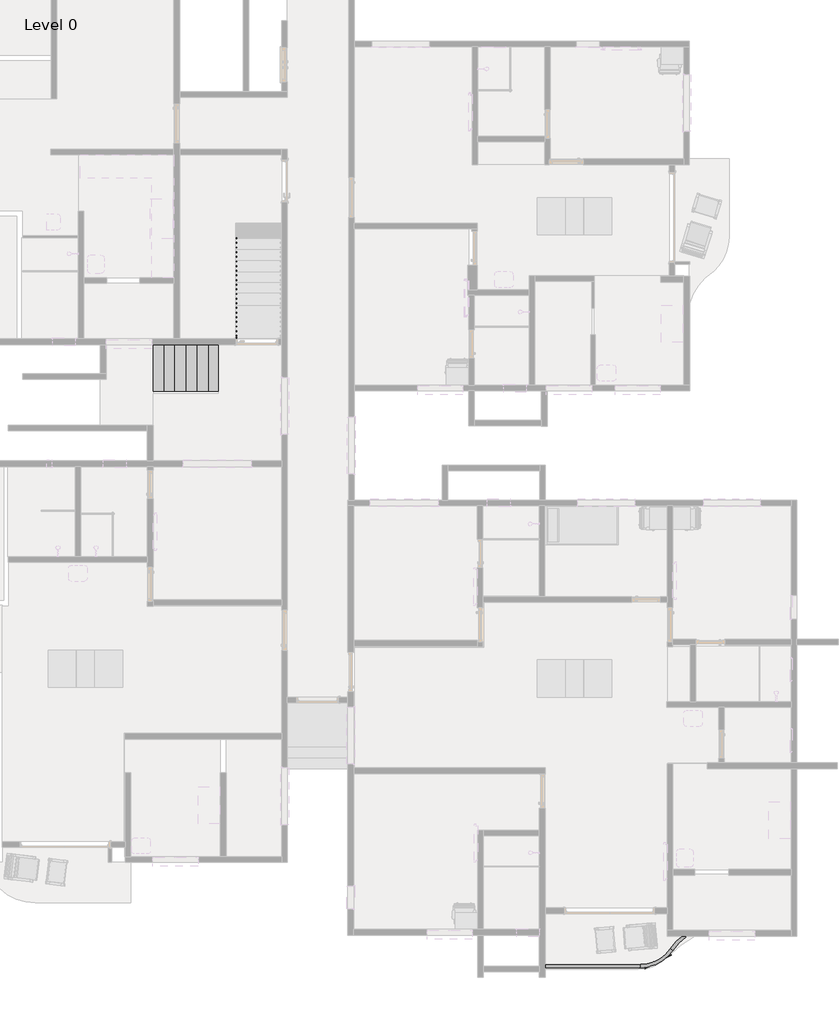
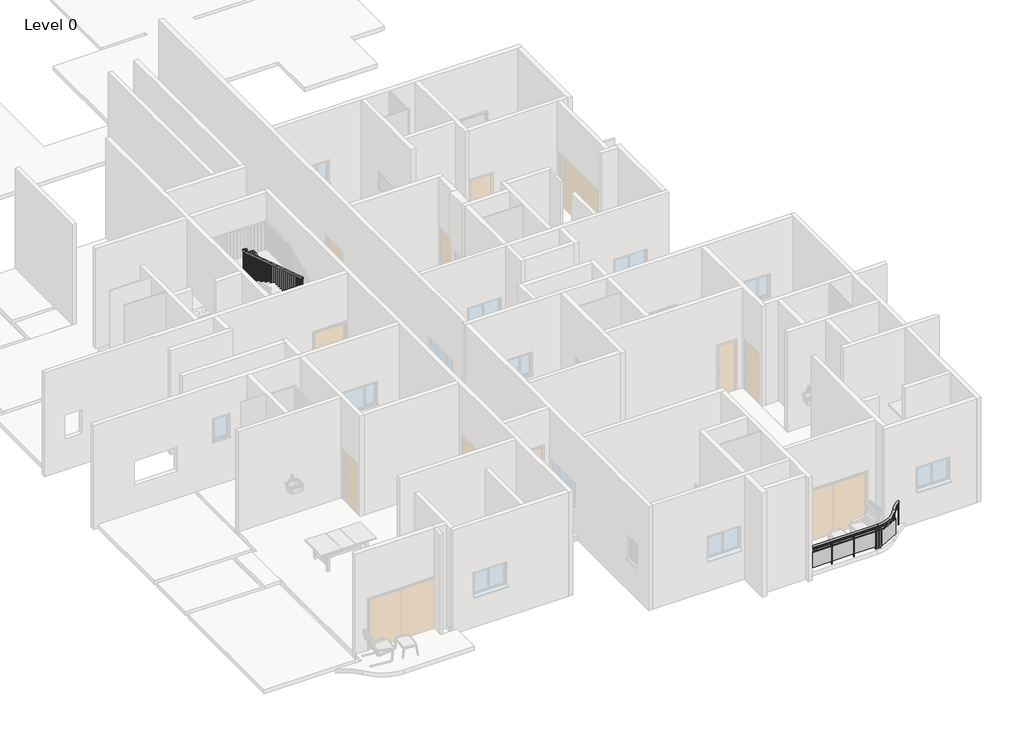
# One storey, part 9 of 14: 2 railings, 1 stair flight.
"""IFC4 building model written with IfcOpenShell, lengths in millimetres."""

from ifc_helpers import new_model, si_unit, point, frame, origin, place, context, project, spatial, polyline, circle_curve, ellipse_curve, trimmed, outline, extrude, faceted_brep, element, save
from ifc_brep_helpers import plane_surface, cylinder_surface, revolved_surface, extruded_surface, advanced_brep

model = new_model("IFC4")

# Units and contexts
model_context = context("Model", 3, world=origin())
ifc_project = project(units=[si_unit("LENGTHUNIT", "METRE", prefix="MILLI")], contexts=[model_context])

# Site, building, storey
site = spatial("IfcSite", under=ifc_project)
building = spatial("IfcBuilding", under=site)
storey = spatial("IfcBuildingStorey", under=building, Name="Level 0", Elevation=0.0)

# Railings
placement = place(None, origin())
element("IfcRailing", 1, ObjectType="1100mm", at=placement, inside=storey, context=model_context, shape_type="SolidModel", body=[
    faceted_brep([(-22988.5547508, 25955.1270746, 1266.6666667), (-22988.5547508, 25955.1270746, 1211.4472941), (-22938.5547508, 25955.1270746, 1211.4472941), (-22938.5547508, 25955.1270746, 1266.6666667), (-22988.5547508, 29511.1270746, 2933.3333333), (-22988.5547508, 29522.2631279, 2883.3333333), (-22938.5547508, 29522.2631279, 2883.3333333), (-22938.5547508, 29511.1270746, 2933.3333333), (-22988.5547508, 29613.1270746, 2933.3333333), (-22988.5547508, 29613.1270746, 2883.3333333), (-22938.5547508, 29663.1270746, 2883.3333333), (-22938.5547508, 29663.1270746, 2933.3333333), (-23193.7547508, 29613.1270746, 2933.3333333), (-23243.7547508, 29613.1270746, 2883.3333333), (-23243.7547508, 29663.1270746, 2883.3333333), (-23193.7547508, 29663.1270746, 2933.3333333), (-23193.7547508, 29613.1270746, 3091.1912752), (-23243.7547508, 29613.1270746, 3041.1912752), (-23243.7547508, 29663.1270746, 3041.1912752), (-23193.7547508, 29663.1270746, 3091.1912752), (-23268.7547508, 29613.1270746, 3091.1912752), (-23268.7547508, 29613.1270746, 3041.1912752), (-23318.7547508, 29663.1270746, 3041.1912752), (-23318.7547508, 29663.1270746, 3091.1912752), (-23268.7547508, 29538.1270746, 3091.1912752), (-23268.7547508, 29530.1770469, 3041.1912752), (-23318.7547508, 29530.1770469, 3041.1912752), (-23318.7547508, 29538.1270746, 3091.1912752), (-23268.7547508, 25935.1270746, 4266.6666667), (-23318.7547508, 25935.1270746, 4266.6666667), (-23318.7547508, 25935.1270746, 4214.0729775), (-23268.7547508, 25935.1270746, 4214.0729775)], [[[0, 1, 2, 3]], [[1, 0, 4, 5]], [[2, 1, 5, 6]], [[3, 2, 6, 7]], [[0, 3, 7, 4]], [[5, 4, 8, 9]], [[6, 5, 9, 10]], [[7, 6, 10, 11]], [[4, 7, 11, 8]], [[9, 8, 12, 13]], [[10, 9, 13, 14]], [[11, 10, 14, 15]], [[8, 11, 15, 12]], [[13, 12, 16, 17]], [[14, 13, 17, 18]], [[15, 14, 18, 19]], [[12, 15, 19, 16]], [[17, 16, 20, 21]], [[18, 17, 21, 22]], [[19, 18, 22, 23]], [[16, 19, 23, 20]], [[21, 20, 24, 25]], [[22, 21, 25, 26]], [[23, 22, 26, 27]], [[20, 23, 27, 24]], [[28, 29, 30, 31]], [[25, 24, 28, 31]], [[26, 25, 31, 30]], [[27, 26, 30, 29]], [[24, 27, 29, 28]]]),
    extrude(outline(polyline([(25963.1270746, 3000.0), (25938.1270746, 3000.0), (25938.1270746, 4213.0942303), (25963.1270746, 4204.9380036), (25963.1270746, 3000.0)])), frame((-23306.2547508, 0.0, 0.0), z_axis=(1.0, 0.0, 0.0), x_axis=(0.0, 1.0, 0.0)), (0.0, 0.0, 1.0), 25.0),
    extrude(outline(polyline([(26088.1270746, 3000.0), (26063.1270746, 3000.0), (26063.1270746, 4172.3130969), (26088.1270746, 4164.1568702), (26088.1270746, 3000.0)])), frame((-23306.2547508, 0.0, 0.0), z_axis=(1.0, 0.0, 0.0), x_axis=(0.0, 1.0, 0.0)), (0.0, 0.0, 1.0), 25.0),
    extrude(outline(polyline([(26213.1270746, 3000.0), (26188.1270746, 3000.0), (26188.1270746, 4131.5319634), (26213.1270746, 4123.3757367), (26213.1270746, 3000.0)])), frame((-23306.2547508, 0.0, 0.0), z_axis=(1.0, 0.0, 0.0), x_axis=(0.0, 1.0, 0.0)), (0.0, 0.0, 1.0), 25.0),
    extrude(outline(polyline([(26338.1270746, 3000.0), (26313.1270746, 3000.0), (26313.1270746, 4090.7508299), (26338.1270746, 4082.5946032), (26338.1270746, 3000.0)])), frame((-23306.2547508, 0.0, 0.0), z_axis=(1.0, 0.0, 0.0), x_axis=(0.0, 1.0, 0.0)), (0.0, 0.0, 1.0), 25.0),
    extrude(outline(polyline([(26463.1270746, 3000.0), (26438.1270746, 3000.0), (26438.1270746, 4049.9696964), (26463.1270746, 4041.8134697), (26463.1270746, 3000.0)])), frame((-23306.2547508, 0.0, 0.0), z_axis=(1.0, 0.0, 0.0), x_axis=(0.0, 1.0, 0.0)), (0.0, 0.0, 1.0), 25.0),
    extrude(outline(polyline([(26588.1270746, 3000.0), (26563.1270746, 3000.0), (26563.1270746, 4009.1885629), (26588.1270746, 4001.0323362), (26588.1270746, 3000.0)])), frame((-23306.2547508, 0.0, 0.0), z_axis=(1.0, 0.0, 0.0), x_axis=(0.0, 1.0, 0.0)), (0.0, 0.0, 1.0), 25.0),
    extrude(outline(polyline([(26713.1270746, 3000.0), (26688.1270746, 3000.0), (26688.1270746, 3968.4074294), (26713.1270746, 3960.2512027), (26713.1270746, 3000.0)])), frame((-23306.2547508, 0.0, 0.0), z_axis=(1.0, 0.0, 0.0), x_axis=(0.0, 1.0, 0.0)), (0.0, 0.0, 1.0), 25.0),
    extrude(outline(polyline([(26838.1270746, 3000.0), (26813.1270746, 3000.0), (26813.1270746, 3927.626296), (26838.1270746, 3919.4700693), (26838.1270746, 3000.0)])), frame((-23306.2547508, 0.0, 0.0), z_axis=(1.0, 0.0, 0.0), x_axis=(0.0, 1.0, 0.0)), (0.0, 0.0, 1.0), 25.0),
    extrude(outline(polyline([(26963.1270746, 3000.0), (26938.1270746, 3000.0), (26938.1270746, 3886.8451625), (26963.1270746, 3878.6889358), (26963.1270746, 3000.0)])), frame((-23306.2547508, 0.0, 0.0), z_axis=(1.0, 0.0, 0.0), x_axis=(0.0, 1.0, 0.0)), (0.0, 0.0, 1.0), 25.0),
    extrude(outline(polyline([(27088.1270746, 3000.0), (27063.1270746, 3000.0), (27063.1270746, 3846.064029), (27088.1270746, 3837.9078023), (27088.1270746, 3000.0)])), frame((-23306.2547508, 0.0, 0.0), z_axis=(1.0, 0.0, 0.0), x_axis=(0.0, 1.0, 0.0)), (0.0, 0.0, 1.0), 25.0),
    extrude(outline(polyline([(27213.1270746, 3000.0), (27188.1270746, 3000.0), (27188.1270746, 3805.2828955), (27213.1270746, 3797.1266688), (27213.1270746, 3000.0)])), frame((-23306.2547508, 0.0, 0.0), z_axis=(1.0, 0.0, 0.0), x_axis=(0.0, 1.0, 0.0)), (0.0, 0.0, 1.0), 25.0),
    extrude(outline(polyline([(27338.1270746, 3000.0), (27313.1270746, 3000.0), (27313.1270746, 3764.501762), (27338.1270746, 3756.3455353), (27338.1270746, 3000.0)])), frame((-23306.2547508, 0.0, 0.0), z_axis=(1.0, 0.0, 0.0), x_axis=(0.0, 1.0, 0.0)), (0.0, 0.0, 1.0), 25.0),
    extrude(outline(polyline([(27463.1270746, 3000.0), (27438.1270746, 3000.0), (27438.1270746, 3723.7206285), (27463.1270746, 3715.5644019), (27463.1270746, 3000.0)])), frame((-23306.2547508, 0.0, 0.0), z_axis=(1.0, 0.0, 0.0), x_axis=(0.0, 1.0, 0.0)), (0.0, 0.0, 1.0), 25.0),
    extrude(outline(polyline([(27588.1270746, 3000.0), (27563.1270746, 3000.0), (27563.1270746, 3682.9394951), (27588.1270746, 3674.7832684), (27588.1270746, 3000.0)])), frame((-23306.2547508, 0.0, 0.0), z_axis=(1.0, 0.0, 0.0), x_axis=(0.0, 1.0, 0.0)), (0.0, 0.0, 1.0), 25.0),
    extrude(outline(polyline([(27713.1270746, 3000.0), (27688.1270746, 3000.0), (27688.1270746, 3642.1583616), (27713.1270746, 3634.0021349), (27713.1270746, 3000.0)])), frame((-23306.2547508, 0.0, 0.0), z_axis=(1.0, 0.0, 0.0), x_axis=(0.0, 1.0, 0.0)), (0.0, 0.0, 1.0), 25.0),
    extrude(outline(polyline([(27838.1270746, 2833.3333333), (27813.1270746, 2833.3333333), (27813.1270746, 3601.3772281), (27838.1270746, 3593.2210014), (27838.1270746, 2833.3333333)])), frame((-23306.2547508, 0.0, 0.0), z_axis=(1.0, 0.0, 0.0), x_axis=(0.0, 1.0, 0.0)), (0.0, 0.0, 1.0), 25.0),
    extrude(outline(polyline([(27963.1270746, 2833.3333333), (27938.1270746, 2833.3333333), (27938.1270746, 3560.5960946), (27963.1270746, 3552.4398679), (27963.1270746, 2833.3333333)])), frame((-23306.2547508, 0.0, 0.0), z_axis=(1.0, 0.0, 0.0), x_axis=(0.0, 1.0, 0.0)), (0.0, 0.0, 1.0), 25.0),
    extrude(outline(polyline([(28088.1270746, 2666.6666667), (28063.1270746, 2666.6666667), (28063.1270746, 3519.8149611), (28088.1270746, 3511.6587344), (28088.1270746, 2666.6666667)])), frame((-23306.2547508, 0.0, 0.0), z_axis=(1.0, 0.0, 0.0), x_axis=(0.0, 1.0, 0.0)), (0.0, 0.0, 1.0), 25.0),
    extrude(outline(polyline([(28213.1270746, 2666.6666667), (28188.1270746, 2666.6666667), (28188.1270746, 3479.0338277), (28213.1270746, 3470.877601), (28213.1270746, 2666.6666667)])), frame((-23306.2547508, 0.0, 0.0), z_axis=(1.0, 0.0, 0.0), x_axis=(0.0, 1.0, 0.0)), (0.0, 0.0, 1.0), 25.0),
    extrude(outline(polyline([(28338.1270746, 2666.6666667), (28313.1270746, 2666.6666667), (28313.1270746, 3438.2526942), (28338.1270746, 3430.0964675), (28338.1270746, 2666.6666667)])), frame((-23306.2547508, 0.0, 0.0), z_axis=(1.0, 0.0, 0.0), x_axis=(0.0, 1.0, 0.0)), (0.0, 0.0, 1.0), 25.0),
    extrude(outline(polyline([(28463.1270746, 2500.0), (28438.1270746, 2500.0), (28438.1270746, 3397.4715607), (28463.1270746, 3389.315334), (28463.1270746, 2500.0)])), frame((-23306.2547508, 0.0, 0.0), z_axis=(1.0, 0.0, 0.0), x_axis=(0.0, 1.0, 0.0)), (0.0, 0.0, 1.0), 25.0),
    extrude(outline(polyline([(28588.1270746, 2500.0), (28563.1270746, 2500.0), (28563.1270746, 3356.6904272), (28588.1270746, 3348.5342005), (28588.1270746, 2500.0)])), frame((-23306.2547508, 0.0, 0.0), z_axis=(1.0, 0.0, 0.0), x_axis=(0.0, 1.0, 0.0)), (0.0, 0.0, 1.0), 25.0),
    extrude(outline(polyline([(28713.1270746, 2333.3333333), (28688.1270746, 2333.3333333), (28688.1270746, 3315.9092937), (28713.1270746, 3307.753067), (28713.1270746, 2333.3333333)])), frame((-23306.2547508, 0.0, 0.0), z_axis=(1.0, 0.0, 0.0), x_axis=(0.0, 1.0, 0.0)), (0.0, 0.0, 1.0), 25.0),
    extrude(outline(polyline([(28838.1270746, 2333.3333333), (28813.1270746, 2333.3333333), (28813.1270746, 3275.1281602), (28838.1270746, 3266.9719335), (28838.1270746, 2333.3333333)])), frame((-23306.2547508, 0.0, 0.0), z_axis=(1.0, 0.0, 0.0), x_axis=(0.0, 1.0, 0.0)), (0.0, 0.0, 1.0), 25.0),
    extrude(outline(polyline([(28963.1270746, 2166.6666667), (28938.1270746, 2166.6666667), (28938.1270746, 3234.3470268), (28963.1270746, 3226.1908001), (28963.1270746, 2166.6666667)])), frame((-23306.2547508, 0.0, 0.0), z_axis=(1.0, 0.0, 0.0), x_axis=(0.0, 1.0, 0.0)), (0.0, 0.0, 1.0), 25.0),
    extrude(outline(polyline([(29088.1270746, 2166.6666667), (29063.1270746, 2166.6666667), (29063.1270746, 3193.5658933), (29088.1270746, 3185.4096666), (29088.1270746, 2166.6666667)])), frame((-23306.2547508, 0.0, 0.0), z_axis=(1.0, 0.0, 0.0), x_axis=(0.0, 1.0, 0.0)), (0.0, 0.0, 1.0), 25.0),
    extrude(outline(polyline([(29213.1270746, 2166.6666667), (29188.1270746, 2166.6666667), (29188.1270746, 3152.7847598), (29213.1270746, 3144.6285331), (29213.1270746, 2166.6666667)])), frame((-23306.2547508, 0.0, 0.0), z_axis=(1.0, 0.0, 0.0), x_axis=(0.0, 1.0, 0.0)), (0.0, 0.0, 1.0), 25.0),
    extrude(outline(polyline([(29338.1270746, 2000.0), (29313.1270746, 2000.0), (29313.1270746, 3112.0036263), (29338.1270746, 3103.8473996), (29338.1270746, 2000.0)])), frame((-23306.2547508, 0.0, 0.0), z_axis=(1.0, 0.0, 0.0), x_axis=(0.0, 1.0, 0.0)), (0.0, 0.0, 1.0), 25.0),
    extrude(outline(polyline([(29463.1270746, 2000.0), (29438.1270746, 2000.0), (29438.1270746, 3071.2224928), (29463.1270746, 3063.0662661), (29463.1270746, 2000.0)])), frame((-23306.2547508, 0.0, 0.0), z_axis=(1.0, 0.0, 0.0), x_axis=(0.0, 1.0, 0.0)), (0.0, 0.0, 1.0), 25.0),
    extrude(outline(polyline([(-23281.2547508, 29588.1270746), (-23281.2547508, 29563.1270746), (-23306.2547508, 29563.1270746), (-23306.2547508, 29588.1270746), (-23281.2547508, 29588.1270746)])), frame((0.0, 0.0, 1833.3333333), z_axis=(0.0, 0.0, 1.0), x_axis=(1.0, 0.0, 0.0)), (0.0, 0.0, 1.0), 1207.8579418),
    extrude(outline(polyline([(-23263.5547508, 29625.6270746), (-23288.5547508, 29625.6270746), (-23288.5547508, 29650.6270746), (-23263.5547508, 29650.6270746), (-23263.5547508, 29625.6270746)])), frame((0.0, 0.0, 1833.3333333), z_axis=(0.0, 0.0, 1.0), x_axis=(1.0, 0.0, 0.0)), (0.0, 0.0, 1.0), 1207.8579418),
    extrude(outline(polyline([(-23138.5547508, 29625.6270746), (-23163.5547508, 29625.6270746), (-23163.5547508, 29650.6270746), (-23138.5547508, 29650.6270746), (-23138.5547508, 29625.6270746)])), frame((0.0, 0.0, 1833.3333333), z_axis=(0.0, 0.0, 1.0), x_axis=(1.0, 0.0, 0.0)), (0.0, 0.0, 1.0), 1050.0),
    extrude(outline(polyline([(-23013.5547508, 29625.6270746), (-23038.5547508, 29625.6270746), (-23038.5547508, 29650.6270746), (-23013.5547508, 29650.6270746), (-23013.5547508, 29625.6270746)])), frame((0.0, 0.0, 1833.3333333), z_axis=(0.0, 0.0, 1.0), x_axis=(1.0, 0.0, 0.0)), (0.0, 0.0, 1.0), 1050.0),
    extrude(outline(polyline([(-22976.0547508, 29505.1270746), (-22976.0547508, 29530.1270746), (-22951.0547508, 29530.1270746), (-22951.0547508, 29505.1270746), (-22976.0547508, 29505.1270746)])), frame((0.0, 0.0, 1833.3333333), z_axis=(0.0, 0.0, 1.0), x_axis=(1.0, 0.0, 0.0)), (0.0, 0.0, 1.0), 1050.0),
    extrude(outline(polyline([(29380.1270746, 2816.7153856), (29405.1270746, 2828.432671), (29405.1270746, 1666.6666667), (29380.1270746, 1666.6666667), (29380.1270746, 2816.7153856)])), frame((-22976.0547508, 0.0, 0.0), z_axis=(1.0, 0.0, 0.0), x_axis=(0.0, 1.0, 0.0)), (0.0, 0.0, 1.0), 25.0),
    extrude(outline(polyline([(29255.1270746, 2758.1289589), (29280.1270746, 2769.8462443), (29280.1270746, 1666.6666667), (29255.1270746, 1666.6666667), (29255.1270746, 2758.1289589)])), frame((-22976.0547508, 0.0, 0.0), z_axis=(1.0, 0.0, 0.0), x_axis=(0.0, 1.0, 0.0)), (0.0, 0.0, 1.0), 25.0),
    extrude(outline(polyline([(29130.1270746, 2699.5425322), (29155.1270746, 2711.2598176), (29155.1270746, 1500.0), (29130.1270746, 1500.0), (29130.1270746, 2699.5425322)])), frame((-22976.0547508, 0.0, 0.0), z_axis=(1.0, 0.0, 0.0), x_axis=(0.0, 1.0, 0.0)), (0.0, 0.0, 1.0), 25.0),
    extrude(outline(polyline([(29005.1270746, 2640.9561055), (29030.1270746, 2652.6733909), (29030.1270746, 1500.0), (29005.1270746, 1500.0), (29005.1270746, 2640.9561055)])), frame((-22976.0547508, 0.0, 0.0), z_axis=(1.0, 0.0, 0.0), x_axis=(0.0, 1.0, 0.0)), (0.0, 0.0, 1.0), 25.0),
    extrude(outline(polyline([(28880.1270746, 2582.3696788), (28905.1270746, 2594.0869642), (28905.1270746, 1333.3333333), (28880.1270746, 1333.3333333), (28880.1270746, 2582.3696788)])), frame((-22976.0547508, 0.0, 0.0), z_axis=(1.0, 0.0, 0.0), x_axis=(0.0, 1.0, 0.0)), (0.0, 0.0, 1.0), 25.0),
    extrude(outline(polyline([(28755.1270746, 2523.7832521), (28780.1270746, 2535.5005375), (28780.1270746, 1333.3333333), (28755.1270746, 1333.3333333), (28755.1270746, 2523.7832521)])), frame((-22976.0547508, 0.0, 0.0), z_axis=(1.0, 0.0, 0.0), x_axis=(0.0, 1.0, 0.0)), (0.0, 0.0, 1.0), 25.0),
    extrude(outline(polyline([(28630.1270746, 2465.1968254), (28655.1270746, 2476.9141108), (28655.1270746, 1166.6666667), (28630.1270746, 1166.6666667), (28630.1270746, 2465.1968254)])), frame((-22976.0547508, 0.0, 0.0), z_axis=(1.0, 0.0, 0.0), x_axis=(0.0, 1.0, 0.0)), (0.0, 0.0, 1.0), 25.0),
    extrude(outline(polyline([(28505.1270746, 2406.6103987), (28530.1270746, 2418.3276841), (28530.1270746, 1166.6666667), (28505.1270746, 1166.6666667), (28505.1270746, 2406.6103987)])), frame((-22976.0547508, 0.0, 0.0), z_axis=(1.0, 0.0, 0.0), x_axis=(0.0, 1.0, 0.0)), (0.0, 0.0, 1.0), 25.0),
    extrude(outline(polyline([(28380.1270746, 2348.023972), (28405.1270746, 2359.7412574), (28405.1270746, 1166.6666667), (28380.1270746, 1166.6666667), (28380.1270746, 2348.023972)])), frame((-22976.0547508, 0.0, 0.0), z_axis=(1.0, 0.0, 0.0), x_axis=(0.0, 1.0, 0.0)), (0.0, 0.0, 1.0), 25.0),
    extrude(outline(polyline([(28255.1270746, 2289.4375454), (28280.1270746, 2301.1548307), (28280.1270746, 1000.0), (28255.1270746, 1000.0), (28255.1270746, 2289.4375454)])), frame((-22976.0547508, 0.0, 0.0), z_axis=(1.0, 0.0, 0.0), x_axis=(0.0, 1.0, 0.0)), (0.0, 0.0, 1.0), 25.0),
    extrude(outline(polyline([(28130.1270746, 2230.8511187), (28155.1270746, 2242.568404), (28155.1270746, 1000.0), (28130.1270746, 1000.0), (28130.1270746, 2230.8511187)])), frame((-22976.0547508, 0.0, 0.0), z_axis=(1.0, 0.0, 0.0), x_axis=(0.0, 1.0, 0.0)), (0.0, 0.0, 1.0), 25.0),
    extrude(outline(polyline([(28005.1270746, 2172.264692), (28030.1270746, 2183.9819773), (28030.1270746, 833.3333333), (28005.1270746, 833.3333333), (28005.1270746, 2172.264692)])), frame((-22976.0547508, 0.0, 0.0), z_axis=(1.0, 0.0, 0.0), x_axis=(0.0, 1.0, 0.0)), (0.0, 0.0, 1.0), 25.0),
    extrude(outline(polyline([(27880.1270746, 2113.6782653), (27905.1270746, 2125.3955506), (27905.1270746, 833.3333333), (27880.1270746, 833.3333333), (27880.1270746, 2113.6782653)])), frame((-22976.0547508, 0.0, 0.0), z_axis=(1.0, 0.0, 0.0), x_axis=(0.0, 1.0, 0.0)), (0.0, 0.0, 1.0), 25.0),
    extrude(outline(polyline([(27755.1270746, 2055.0918386), (27780.1270746, 2066.8091239), (27780.1270746, 833.3333333), (27755.1270746, 833.3333333), (27755.1270746, 2055.0918386)])), frame((-22976.0547508, 0.0, 0.0), z_axis=(1.0, 0.0, 0.0), x_axis=(0.0, 1.0, 0.0)), (0.0, 0.0, 1.0), 25.0),
    extrude(outline(polyline([(27630.1270746, 1996.5054119), (27655.1270746, 2008.2226972), (27655.1270746, 666.6666667), (27630.1270746, 666.6666667), (27630.1270746, 1996.5054119)])), frame((-22976.0547508, 0.0, 0.0), z_axis=(1.0, 0.0, 0.0), x_axis=(0.0, 1.0, 0.0)), (0.0, 0.0, 1.0), 25.0),
    extrude(outline(polyline([(27505.1270746, 1937.9189852), (27530.1270746, 1949.6362705), (27530.1270746, 666.6666667), (27505.1270746, 666.6666667), (27505.1270746, 1937.9189852)])), frame((-22976.0547508, 0.0, 0.0), z_axis=(1.0, 0.0, 0.0), x_axis=(0.0, 1.0, 0.0)), (0.0, 0.0, 1.0), 25.0),
    extrude(outline(polyline([(27380.1270746, 1879.3325585), (27405.1270746, 1891.0498438), (27405.1270746, 500.0), (27380.1270746, 500.0), (27380.1270746, 1879.3325585)])), frame((-22976.0547508, 0.0, 0.0), z_axis=(1.0, 0.0, 0.0), x_axis=(0.0, 1.0, 0.0)), (0.0, 0.0, 1.0), 25.0),
    extrude(outline(polyline([(27255.1270746, 1820.7461318), (27280.1270746, 1832.4634171), (27280.1270746, 500.0), (27255.1270746, 500.0), (27255.1270746, 1820.7461318)])), frame((-22976.0547508, 0.0, 0.0), z_axis=(1.0, 0.0, 0.0), x_axis=(0.0, 1.0, 0.0)), (0.0, 0.0, 1.0), 25.0),
    extrude(outline(polyline([(27130.1270746, 1762.1597051), (27155.1270746, 1773.8769904), (27155.1270746, 333.3333333), (27130.1270746, 333.3333333), (27130.1270746, 1762.1597051)])), frame((-22976.0547508, 0.0, 0.0), z_axis=(1.0, 0.0, 0.0), x_axis=(0.0, 1.0, 0.0)), (0.0, 0.0, 1.0), 25.0),
    extrude(outline(polyline([(27005.1270746, 1703.5732784), (27030.1270746, 1715.2905637), (27030.1270746, 333.3333333), (27005.1270746, 333.3333333), (27005.1270746, 1703.5732784)])), frame((-22976.0547508, 0.0, 0.0), z_axis=(1.0, 0.0, 0.0), x_axis=(0.0, 1.0, 0.0)), (0.0, 0.0, 1.0), 25.0),
    extrude(outline(polyline([(26880.1270746, 1644.9868517), (26905.1270746, 1656.704137), (26905.1270746, 333.3333333), (26880.1270746, 333.3333333), (26880.1270746, 1644.9868517)])), frame((-22976.0547508, 0.0, 0.0), z_axis=(1.0, 0.0, 0.0), x_axis=(0.0, 1.0, 0.0)), (0.0, 0.0, 1.0), 25.0),
    extrude(outline(polyline([(26755.1270746, 1586.400425), (26780.1270746, 1598.1177103), (26780.1270746, 166.6666667), (26755.1270746, 166.6666667), (26755.1270746, 1586.400425)])), frame((-22976.0547508, 0.0, 0.0), z_axis=(1.0, 0.0, 0.0), x_axis=(0.0, 1.0, 0.0)), (0.0, 0.0, 1.0), 25.0),
    extrude(outline(polyline([(26630.1270746, 1527.8139983), (26655.1270746, 1539.5312836), (26655.1270746, 166.6666667), (26630.1270746, 166.6666667), (26630.1270746, 1527.8139983)])), frame((-22976.0547508, 0.0, 0.0), z_axis=(1.0, 0.0, 0.0), x_axis=(0.0, 1.0, 0.0)), (0.0, 0.0, 1.0), 25.0),
    extrude(outline(polyline([(26505.1270746, 1469.2275716), (26530.1270746, 1480.9448569), (26530.1270746, 166.6666667), (26505.1270746, 166.6666667), (26505.1270746, 1469.2275716)])), frame((-22976.0547508, 0.0, 0.0), z_axis=(1.0, 0.0, 0.0), x_axis=(0.0, 1.0, 0.0)), (0.0, 0.0, 1.0), 25.0),
    extrude(outline(polyline([(26380.1270746, 1410.6411449), (26405.1270746, 1422.3584302), (26405.1270746, 166.6666667), (26380.1270746, 166.6666667), (26380.1270746, 1410.6411449)])), frame((-22976.0547508, 0.0, 0.0), z_axis=(1.0, 0.0, 0.0), x_axis=(0.0, 1.0, 0.0)), (0.0, 0.0, 1.0), 25.0),
    extrude(outline(polyline([(26255.1270746, 1352.0547182), (26280.1270746, 1363.7720035), (26280.1270746, 166.6666667), (26255.1270746, 166.6666667), (26255.1270746, 1352.0547182)])), frame((-22976.0547508, 0.0, 0.0), z_axis=(1.0, 0.0, 0.0), x_axis=(0.0, 1.0, 0.0)), (0.0, 0.0, 1.0), 25.0),
    extrude(outline(polyline([(26130.1270746, 1293.4682915), (26155.1270746, 1305.1855768), (26155.1270746, 166.6666667), (26130.1270746, 166.6666667), (26130.1270746, 1293.4682915)])), frame((-22976.0547508, 0.0, 0.0), z_axis=(1.0, 0.0, 0.0), x_axis=(0.0, 1.0, 0.0)), (0.0, 0.0, 1.0), 25.0),
    extrude(outline(polyline([(26005.1270746, 1234.8818648), (26030.1270746, 1246.5991502), (26030.1270746, 166.6666667), (26005.1270746, 166.6666667), (26005.1270746, 1234.8818648)])), frame((-22976.0547508, 0.0, 0.0), z_axis=(1.0, 0.0, 0.0), x_axis=(0.0, 1.0, 0.0)), (0.0, 0.0, 1.0), 25.0),
    extrude(outline(polyline([(-23281.2547508, 29625.6270746), (-23306.2547508, 29625.6270746), (-23306.2547508, 29650.6270746), (-23281.2547508, 29650.6270746), (-23281.2547508, 29625.6270746)])), frame((0.0, 0.0, 1833.3333333), z_axis=(0.0, 0.0, 1.0), x_axis=(1.0, 0.0, 0.0)), (0.0, 0.0, 1.0), 1207.8579418),
    extrude(outline(polyline([(-22976.0547508, 29625.6270746), (-22976.0547508, 29650.6270746), (-22951.0547508, 29650.6270746), (-22951.0547508, 29625.6270746), (-22976.0547508, 29625.6270746)])), frame((0.0, 0.0, 1833.3333333), z_axis=(0.0, 0.0, 1.0), x_axis=(1.0, 0.0, 0.0)), (0.0, 0.0, 1.0), 1050.0),
    extrude(outline(polyline([(25960.1270746, 3000.0), (25935.1270746, 3000.0), (25935.1270746, 4214.0729775), (25960.1270746, 4205.9167508), (25960.1270746, 3000.0)])), frame((-23306.2547508, 0.0, 0.0), z_axis=(1.0, 0.0, 0.0), x_axis=(0.0, 1.0, 0.0)), (0.0, 0.0, 1.0), 25.0),
    extrude(outline(polyline([(25955.1270746, 1211.4472941), (25980.1270746, 1223.1645795), (25980.1270746, 166.6666667), (25955.1270746, 166.6666667), (25955.1270746, 1211.4472941)])), frame((-22976.0547508, 0.0, 0.0), z_axis=(1.0, 0.0, 0.0), x_axis=(0.0, 1.0, 0.0)), (0.0, 0.0, 1.0), 25.0),
])
element("IfcRailing", 2, ObjectType="Glass_Panel-Bottom_Fill", at=placement, inside=storey, context=model_context, shape_type="SolidModel", body=[
    advanced_brep(
    [(-14663.0433343, 9103.6906738, 1049.9616), (-14663.0433343, 9023.6906738, 1049.9616), (-12097.6433343, 9103.6906738, 1049.9616), (-12097.6433343, 9023.6906738, 1049.9616), (-11234.1826051, 9482.8008874, 1049.9616), (-11300.5056109, 9527.5363197, 1049.9616), (-10876.9280101, 9840.0554824, 1049.9616), (-10921.6634424, 9906.3784882, 1049.9616)],
    [
        (0, 1, ellipse_curve(frame((-14663.0433343, 9063.6906738, 1049.9616), z_axis=(-1.0, 0.0, 0.0), x_axis=(0.0, -1.0, 0.0)), 40.0, 30.0)),
        (1, 0, ellipse_curve(frame((-14663.0433343, 9063.6906738, 1049.9616), z_axis=(-1.0, 0.0, 0.0), x_axis=(0.0, -1.0, 0.0)), 40.0, 30.0)),
        (0, 2),
        (2, 3, ellipse_curve(frame((-12097.6433343, 9063.6906738, 1049.9616), z_axis=(-1.0, 0.0, 0.0), x_axis=(0.0, -1.0, 0.0)), 40.0, 30.0)),
        (3, 1),
        (3, 2, ellipse_curve(frame((-12097.6433343, 9063.6906738, 1049.9616), z_axis=(-1.0, 0.0, 0.0), x_axis=(0.0, -1.0, 0.0)), 40.0, 30.0)),
        (4, 3, circle_curve(frame((-12097.6433343, 10065.2125033, 1049.9616), z_axis=(0.0, 0.0, -1.0), x_axis=(0.0, -1.0, 0.0)), 1041.5218294)),
        (2, 5, circle_curve(frame((-12097.6433343, 10065.2125033, 1049.9616), z_axis=(0.0, 0.0, 1.0), x_axis=(0.0, -1.0, 0.0)), 961.5218294)),
        (5, 4, ellipse_curve(frame((-11267.344108, 9505.1686036, 1049.9616), z_axis=(-0.5591929034707565, -0.8290375725550352, 0.0), x_axis=(0.8290375725550352, -0.5591929034707565, 0.0)), 40.0, 30.0)),
        (4, 5, ellipse_curve(frame((-11267.344108, 9505.1686036, 1049.9616), z_axis=(-0.559192903470757, -0.8290375725550349, 0.0), x_axis=(0.8290375725550349, -0.559192903470757, 0.0)), 40.0, 30.0)),
        (6, 4, circle_curve(frame((-10136.5975269, 8742.4704043, 1049.9616), z_axis=(0.0, 0.0, 1.0), x_axis=(-0.8290375725550352, 0.5591929034707565, 0.0)), 1323.9268212)),
        (5, 7, circle_curve(frame((-10136.5975269, 8742.4704043, 1049.9616), z_axis=(0.0, 0.0, -1.0), x_axis=(-0.8290375725550352, 0.5591929034707565, 0.0)), 1403.9268212)),
        (7, 6, ellipse_curve(frame((-10899.2957262, 9873.2169853, 1049.9616), z_axis=(-0.8290375725550363, -0.5591929034707548, 0.0), x_axis=(0.5591929034707548, -0.8290375725550363, 0.0)), 40.0, 30.0)),
        (6, 7, ellipse_curve(frame((-10899.2957262, 9873.2169853, 1049.9616), z_axis=(-0.8290375725550369, -0.5591929034707543, 0.0), x_axis=(0.5591929034707542, -0.8290375725550366, 0.0)), 40.0, 30.0)),
    ],
    [
        plane_surface(frame((-14663.0433343, 9063.6906738, 1049.9616), z_axis=(-1.0, 0.0, 0.0), x_axis=(0.0, 1.0, 0.0))),
        extruded_surface(trimmed(ellipse_curve(frame((-12097.6433343, 9063.6906738, 1049.9616), z_axis=(-1.0, 0.0, 0.0), x_axis=(0.0, -1.0, 0.0)), 40.0, 30.0), [point((-12097.6433343, 9103.6906738, 1049.9616))], [point((-12097.6433343, 9023.6906738, 1049.9616))], True, "CARTESIAN"), (-2565.3999999999996, 0.0, 0.0), 2565.3999999999996),
        extruded_surface(trimmed(ellipse_curve(frame((-12097.6433343, 9063.6906738, 1049.9616), z_axis=(-1.0, 0.0, 0.0), x_axis=(0.0, -1.0, 0.0)), 40.0, 30.0), [point((-12097.6433343, 9023.6906738, 1049.9616))], [point((-12097.6433343, 9103.6906738, 1049.9616))], True, "CARTESIAN"), (-2565.3999999999996, 0.0, 0.0), 2565.3999999999996),
        revolved_surface(trimmed(ellipse_curve(frame((-12097.6433343, 9063.6906738, 1049.9616), z_axis=(-1.0, 0.0, 0.0), x_axis=(0.0, -1.0, 0.0)), 40.0, 30.0), [point((-12097.6433343, 9103.6906738, 1049.9616))], [point((-12097.6433343, 9023.6906738, 1049.9616))], True, "CARTESIAN"), (-12097.6433343, 10065.2125033, 1049.9616), (0.0, 0.0, 1.0)),
        revolved_surface(trimmed(ellipse_curve(frame((-12097.6433343, 9063.6906738, 1049.9616), z_axis=(-1.0, 0.0, 0.0), x_axis=(0.0, -1.0, 0.0)), 40.0, 30.0), [point((-12097.6433343, 9023.6906738, 1049.9616))], [point((-12097.6433343, 9103.6906738, 1049.9616))], True, "CARTESIAN"), (-12097.6433343, 10065.2125033, 1049.9616), (0.0, 0.0, 1.0)),
        revolved_surface(trimmed(ellipse_curve(frame((-11267.344108, 9505.1686036, 1049.9616), z_axis=(-0.5591929034707565, -0.8290375725550352, 0.0), x_axis=(0.8290375725550352, -0.5591929034707565, 0.0)), 40.0, 30.0), [point((-11300.5056109, 9527.5363197, 1049.9616))], [point((-11234.1826051, 9482.8008874, 1049.9616))], True, "CARTESIAN"), (-10136.5975269, 8742.4704043, 1049.9616), (0.0, 0.0, -1.0)),
        revolved_surface(trimmed(ellipse_curve(frame((-11267.344108, 9505.1686036, 1049.9616), z_axis=(-0.5591929034707565, -0.8290375725550352, 0.0), x_axis=(0.8290375725550352, -0.5591929034707565, 0.0)), 40.0, 30.0), [point((-11234.1826051, 9482.8008874, 1049.9616))], [point((-11300.5056109, 9527.5363197, 1049.9616))], True, "CARTESIAN"), (-10136.5975269, 8742.4704043, 1049.9616), (0.0, 0.0, -1.0)),
        plane_surface(frame((-10899.2957262, 9873.2169853, 1049.9616), z_axis=(0.8290375725550365, 0.5591929034707545, 0.0), x_axis=(0.5591929034707545, -0.8290375725550365, 0.0))),
    ],
    [
        (0, [[1, 2]]),
        (1, [[-1, 3, 4, 5]]),
        (2, [[-2, -5, 6, -3]]),
        (3, [[7, -4, 8, 9]]),
        (4, [[-8, -6, -7, 10]]),
        (5, [[11, -9, 12, 13]]),
        (6, [[-12, -10, -11, 14]]),
        (7, [[-14, -13]]),
    ],
),
    advanced_brep(
    [(-14663.0433343, 9054.2999087, 949.9616), (-14663.0433343, 9074.2999087, 949.9616), (-14663.0433343, 9074.2999087, 929.9616), (-14663.0433343, 9054.2999087, 929.9616), (-12097.6433343, 9054.2999087, 949.9616), (-12097.6433343, 9074.2999087, 949.9616), (-12097.6433343, 9074.2999087, 929.9616), (-12097.6433343, 9054.2999087, 929.9616), (-11276.1395623, 9511.1012124, 949.9616), (-11259.5588108, 9499.9173543, 949.9616), (-11276.1395623, 9511.1012124, 929.9616), (-11259.5588108, 9499.9173543, 929.9616), (-10905.2283351, 9882.0124396, 949.9616), (-10894.044477, 9865.4316882, 949.9616), (-10905.2283351, 9882.0124396, 929.9616), (-10894.044477, 9865.4316882, 929.9616)],
    [
        (0, 1),
        (1, 2),
        (2, 3),
        (3, 0),
        (0, 4),
        (4, 5),
        (5, 1),
        (5, 6),
        (6, 2),
        (6, 7),
        (7, 3),
        (7, 4),
        (8, 5, circle_curve(frame((-12097.6433343, 10065.2125033, 949.9616), z_axis=(0.0, 0.0, -1.0), x_axis=(0.0, -1.0, 0.0)), 990.9125946)),
        (4, 9, circle_curve(frame((-12097.6433343, 10065.2125033, 949.9616), z_axis=(0.0, 0.0, 1.0), x_axis=(0.0, -1.0, 0.0)), 1010.9125946)),
        (9, 8),
        (10, 6, circle_curve(frame((-12097.6433343, 10065.2125033, 929.9616), z_axis=(0.0, 0.0, -1.0), x_axis=(0.0, -1.0, 0.0)), 990.9125946)),
        (8, 10),
        (11, 7, circle_curve(frame((-12097.6433343, 10065.2125033, 929.9616), z_axis=(0.0, 0.0, -1.0), x_axis=(0.0, -1.0, 0.0)), 1010.9125946)),
        (10, 11),
        (11, 9),
        (12, 8, circle_curve(frame((-10136.5975269, 8742.4704043, 949.9616), z_axis=(0.0, 0.0, 1.0), x_axis=(-0.8290375725550352, 0.5591929034707565, 0.0)), 1374.5360561)),
        (9, 13, circle_curve(frame((-10136.5975269, 8742.4704043, 949.9616), z_axis=(0.0, 0.0, -1.0), x_axis=(-0.8290375725550352, 0.5591929034707565, 0.0)), 1354.5360561)),
        (13, 12),
        (14, 10, circle_curve(frame((-10136.5975269, 8742.4704043, 929.9616), z_axis=(0.0, 0.0, 1.0), x_axis=(-0.8290375725550352, 0.5591929034707565, 0.0)), 1374.5360561)),
        (12, 14),
        (15, 11, circle_curve(frame((-10136.5975269, 8742.4704043, 929.9616), z_axis=(0.0, 0.0, 1.0), x_axis=(-0.8290375725550352, 0.5591929034707565, 0.0)), 1354.5360561)),
        (14, 15),
        (15, 13),
    ],
    [
        plane_surface(frame((-14663.0433343, 9064.2999087, 949.9616), z_axis=(-1.0, 0.0, 0.0), x_axis=(0.0, 1.0, 0.0))),
        plane_surface(frame((-14663.0433343, 9054.2999087, 949.9616), z_axis=(0.0, 0.0, 1.0), x_axis=(1.0, 0.0, 0.0))),
        plane_surface(frame((-14663.0433343, 9074.2999087, 949.9616), z_axis=(0.0, 1.0, 0.0), x_axis=(1.0, 0.0, 0.0))),
        plane_surface(frame((-14663.0433343, 9074.2999087, 929.9616), z_axis=(0.0, 0.0, -1.0), x_axis=(1.0, 0.0, 0.0))),
        plane_surface(frame((-14663.0433343, 9054.2999087, 929.9616), z_axis=(0.0, -1.0, 0.0), x_axis=(1.0, 0.0, 0.0))),
        plane_surface(frame((-12097.6433343, 10065.2125033, 949.9616), z_axis=(0.0, 0.0, 1.0), x_axis=(0.0, -1.0, 0.0))),
        revolved_surface(polyline([(-12097.6433343, 9074.299908699999, 949.9616), (-12097.6433343, 9074.299908699999, 929.9616)]), (-12097.6433343, 10065.2125033, 949.9616), (0.0, 0.0, 1.0)),
        plane_surface(frame((-12097.6433343, 10065.2125033, 929.9616), z_axis=(0.0, 0.0, -1.0), x_axis=(0.0, -1.0, 0.0))),
        cylinder_surface(frame((-12097.6433343, 10065.2125033, 949.9616), z_axis=(0.0, 0.0, 1.0), x_axis=(0.0, -1.0, 0.0)), 1010.9125946),
        plane_surface(frame((-10136.5975269, 8742.4704043, 949.9616), z_axis=(0.0, 0.0, 1.0), x_axis=(-0.8290375725550352, 0.5591929034707565, 0.0))),
        cylinder_surface(frame((-10136.5975269, 8742.4704043, 949.9616), z_axis=(0.0, 0.0, -1.0), x_axis=(-0.8290375725550352, 0.5591929034707565, 0.0)), 1374.5360561),
        plane_surface(frame((-10136.5975269, 8742.4704043, 929.9616), z_axis=(0.0, 0.0, -1.0), x_axis=(-0.8290375725550352, 0.5591929034707565, 0.0))),
        revolved_surface(polyline([(-11259.558810787414, 9499.917354366387, 929.9616), (-11259.558810787414, 9499.917354366387, 949.9616)]), (-10136.5975269, 8742.4704043, 949.9616), (0.0, 0.0, -1.0)),
        plane_surface(frame((-10899.636406, 9873.7220639, 949.9616), z_axis=(0.8290375725550365, 0.5591929034707545, 0.0), x_axis=(0.5591929034707545, -0.8290375725550365, 0.0))),
    ],
    [
        (0, [[1, 2, 3, 4]]),
        (1, [[-1, 5, 6, 7]]),
        (2, [[-2, -7, 8, 9]]),
        (3, [[-3, -9, 10, 11]]),
        (4, [[-4, -11, 12, -5]]),
        (5, [[13, -6, 14, 15]]),
        (6, [[16, -8, -13, 17]]),
        (7, [[18, -10, -16, 19]]),
        (8, [[-14, -12, -18, 20]]),
        (9, [[21, -15, 22, 23]]),
        (10, [[24, -17, -21, 25]]),
        (11, [[26, -19, -24, 27]]),
        (12, [[-22, -20, -26, 28]]),
        (13, [[-28, -27, -25, -23]]),
    ],
),
    advanced_brep(
    [(-14663.0433343, 9054.2999087, 849.9616), (-14663.0433343, 9074.2999087, 849.9616), (-14663.0433343, 9074.2999087, 829.9616), (-14663.0433343, 9054.2999087, 829.9616), (-12097.6433343, 9054.2999087, 849.9616), (-12097.6433343, 9074.2999087, 849.9616), (-12097.6433343, 9074.2999087, 829.9616), (-12097.6433343, 9054.2999087, 829.9616), (-11276.1395623, 9511.1012124, 849.9616), (-11259.5588108, 9499.9173543, 849.9616), (-11276.1395623, 9511.1012124, 829.9616), (-11259.5588108, 9499.9173543, 829.9616), (-10905.2283351, 9882.0124396, 849.9616), (-10894.044477, 9865.4316882, 849.9616), (-10905.2283351, 9882.0124396, 829.9616), (-10894.044477, 9865.4316882, 829.9616)],
    [
        (0, 1),
        (1, 2),
        (2, 3),
        (3, 0),
        (0, 4),
        (4, 5),
        (5, 1),
        (5, 6),
        (6, 2),
        (6, 7),
        (7, 3),
        (7, 4),
        (8, 5, circle_curve(frame((-12097.6433343, 10065.2125033, 849.9616), z_axis=(0.0, 0.0, -1.0), x_axis=(0.0, -1.0, 0.0)), 990.9125946)),
        (4, 9, circle_curve(frame((-12097.6433343, 10065.2125033, 849.9616), z_axis=(0.0, 0.0, 1.0), x_axis=(0.0, -1.0, 0.0)), 1010.9125946)),
        (9, 8),
        (10, 6, circle_curve(frame((-12097.6433343, 10065.2125033, 829.9616), z_axis=(0.0, 0.0, -1.0), x_axis=(0.0, -1.0, 0.0)), 990.9125946)),
        (8, 10),
        (11, 7, circle_curve(frame((-12097.6433343, 10065.2125033, 829.9616), z_axis=(0.0, 0.0, -1.0), x_axis=(0.0, -1.0, 0.0)), 1010.9125946)),
        (10, 11),
        (11, 9),
        (12, 8, circle_curve(frame((-10136.5975269, 8742.4704043, 849.9616), z_axis=(0.0, 0.0, 1.0), x_axis=(-0.8290375725550352, 0.5591929034707565, 0.0)), 1374.5360561)),
        (9, 13, circle_curve(frame((-10136.5975269, 8742.4704043, 849.9616), z_axis=(0.0, 0.0, -1.0), x_axis=(-0.8290375725550352, 0.5591929034707565, 0.0)), 1354.5360561)),
        (13, 12),
        (14, 10, circle_curve(frame((-10136.5975269, 8742.4704043, 829.9616), z_axis=(0.0, 0.0, 1.0), x_axis=(-0.8290375725550352, 0.5591929034707565, 0.0)), 1374.5360561)),
        (12, 14),
        (15, 11, circle_curve(frame((-10136.5975269, 8742.4704043, 829.9616), z_axis=(0.0, 0.0, 1.0), x_axis=(-0.8290375725550352, 0.5591929034707565, 0.0)), 1354.5360561)),
        (14, 15),
        (15, 13),
    ],
    [
        plane_surface(frame((-14663.0433343, 9064.2999087, 849.9616), z_axis=(-1.0, 0.0, 0.0), x_axis=(0.0, 1.0, 0.0))),
        plane_surface(frame((-14663.0433343, 9054.2999087, 849.9616), z_axis=(0.0, 0.0, 1.0), x_axis=(1.0, 0.0, 0.0))),
        plane_surface(frame((-14663.0433343, 9074.2999087, 849.9616), z_axis=(0.0, 1.0, 0.0), x_axis=(1.0, 0.0, 0.0))),
        plane_surface(frame((-14663.0433343, 9074.2999087, 829.9616), z_axis=(0.0, 0.0, -1.0), x_axis=(1.0, 0.0, 0.0))),
        plane_surface(frame((-14663.0433343, 9054.2999087, 829.9616), z_axis=(0.0, -1.0, 0.0), x_axis=(1.0, 0.0, 0.0))),
        plane_surface(frame((-12097.6433343, 10065.2125033, 849.9616), z_axis=(0.0, 0.0, 1.0), x_axis=(0.0, -1.0, 0.0))),
        revolved_surface(polyline([(-12097.6433343, 9074.299908699999, 849.9616), (-12097.6433343, 9074.299908699999, 829.9616)]), (-12097.6433343, 10065.2125033, 849.9616), (0.0, 0.0, 1.0)),
        plane_surface(frame((-12097.6433343, 10065.2125033, 829.9616), z_axis=(0.0, 0.0, -1.0), x_axis=(0.0, -1.0, 0.0))),
        cylinder_surface(frame((-12097.6433343, 10065.2125033, 849.9616), z_axis=(0.0, 0.0, 1.0), x_axis=(0.0, -1.0, 0.0)), 1010.9125946),
        plane_surface(frame((-10136.5975269, 8742.4704043, 849.9616), z_axis=(0.0, 0.0, 1.0), x_axis=(-0.8290375725550352, 0.5591929034707565, 0.0))),
        cylinder_surface(frame((-10136.5975269, 8742.4704043, 849.9616), z_axis=(0.0, 0.0, -1.0), x_axis=(-0.8290375725550352, 0.5591929034707565, 0.0)), 1374.5360561),
        plane_surface(frame((-10136.5975269, 8742.4704043, 829.9616), z_axis=(0.0, 0.0, -1.0), x_axis=(-0.8290375725550352, 0.5591929034707565, 0.0))),
        revolved_surface(polyline([(-11259.558810787414, 9499.917354366387, 829.9616), (-11259.558810787414, 9499.917354366387, 849.9616)]), (-10136.5975269, 8742.4704043, 849.9616), (0.0, 0.0, -1.0)),
        plane_surface(frame((-10899.636406, 9873.7220639, 849.9616), z_axis=(0.8290375725550365, 0.5591929034707545, 0.0), x_axis=(0.5591929034707545, -0.8290375725550365, 0.0))),
    ],
    [
        (0, [[1, 2, 3, 4]]),
        (1, [[-1, 5, 6, 7]]),
        (2, [[-2, -7, 8, 9]]),
        (3, [[-3, -9, 10, 11]]),
        (4, [[-4, -11, 12, -5]]),
        (5, [[13, -6, 14, 15]]),
        (6, [[16, -8, -13, 17]]),
        (7, [[18, -10, -16, 19]]),
        (8, [[-14, -12, -18, 20]]),
        (9, [[21, -15, 22, 23]]),
        (10, [[24, -17, -21, 25]]),
        (11, [[26, -19, -24, 27]]),
        (12, [[-22, -20, -26, 28]]),
        (13, [[-28, -27, -25, -23]]),
    ],
),
    extrude(outline(polyline([(-11344.1018979, 9445.0377731), (-11336.5333682, 9454.3499886), (-11297.7324702, 9422.8144482), (-11305.3009999, 9413.5022326), (-11344.1018979, 9445.0377731)])), frame((0.0, 0.0, 149.9616), z_axis=(0.0, 0.0, 1.0), x_axis=(1.0, 0.0, 0.0)), (0.0, 0.0, 1.0), 870.0),
    extrude(outline(polyline([(-11980.1126222, 8992.1475952), (-11273.7545479, 9367.7248454), (-11271.4071901, 9363.3101074), (-11977.7652643, 8987.7328572), (-11980.1126222, 8992.1475952)])), frame((0.0, 0.0, 249.9616), z_axis=(0.0, 0.0, 1.0), x_axis=(1.0, 0.0, 0.0)), (0.0, 0.0, 1.0), 580.0),
    extrude(outline(polyline([(-12016.8226498, 9092.6337613), (-12004.8702051, 9093.701032), (-12000.423244, 9043.8991793), (-12012.3756887, 9042.8319086), (-12016.8226498, 9092.6337613)])), frame((0.0, 0.0, 149.9616), z_axis=(0.0, 0.0, 1.0), x_axis=(1.0, 0.0, 0.0)), (0.0, 0.0, 1.0), 870.0),
    extrude(outline(polyline([(-12186.3433343, 9089.2999087), (-12174.3433343, 9089.2999087), (-12174.3433343, 9039.2999087), (-12186.3433343, 9039.2999087), (-12186.3433343, 9089.2999087)])), frame((0.0, 0.0, 149.9616), z_axis=(0.0, 0.0, 1.0), x_axis=(1.0, 0.0, 0.0)), (0.0, 0.0, 1.0), 870.0),
    extrude(outline(polyline([(-12980.3433343, 9062.5750986), (-12180.3433343, 9062.5750986), (-12180.3433343, 9057.5750986), (-12980.3433343, 9057.5750986), (-12980.3433343, 9062.5750986)])), frame((0.0, 0.0, 249.9616), z_axis=(0.0, 0.0, 1.0), x_axis=(1.0, 0.0, 0.0)), (0.0, 0.0, 1.0), 580.0),
    extrude(outline(polyline([(-12986.3433343, 9089.2999087), (-12974.3433343, 9089.2999087), (-12974.3433343, 9039.2999087), (-12986.3433343, 9039.2999087), (-12986.3433343, 9089.2999087)])), frame((0.0, 0.0, 149.9616), z_axis=(0.0, 0.0, 1.0), x_axis=(1.0, 0.0, 0.0)), (0.0, 0.0, 1.0), 870.0),
    extrude(outline(polyline([(-13780.3433343, 9062.5750986), (-12980.3433343, 9062.5750986), (-12980.3433343, 9057.5750986), (-13780.3433343, 9057.5750986), (-13780.3433343, 9062.5750986)])), frame((0.0, 0.0, 249.9616), z_axis=(0.0, 0.0, 1.0), x_axis=(1.0, 0.0, 0.0)), (0.0, 0.0, 1.0), 580.0),
    extrude(outline(polyline([(-13786.3433343, 9089.2999087), (-13774.3433343, 9089.2999087), (-13774.3433343, 9039.2999087), (-13786.3433343, 9039.2999087), (-13786.3433343, 9089.2999087)])), frame((0.0, 0.0, 149.9616), z_axis=(0.0, 0.0, 1.0), x_axis=(1.0, 0.0, 0.0)), (0.0, 0.0, 1.0), 870.0),
    extrude(outline(polyline([(-14580.3433343, 9062.5750986), (-13780.3433343, 9062.5750986), (-13780.3433343, 9057.5750986), (-14580.3433343, 9057.5750986), (-14580.3433343, 9062.5750986)])), frame((0.0, 0.0, 249.9616), z_axis=(0.0, 0.0, 1.0), x_axis=(1.0, 0.0, 0.0)), (0.0, 0.0, 1.0), 580.0),
    extrude(outline(polyline([(-14586.3433343, 9089.2999087), (-14574.3433343, 9089.2999087), (-14574.3433343, 9039.2999087), (-14586.3433343, 9039.2999087), (-14586.3433343, 9089.2999087)])), frame((0.0, 0.0, 149.9616), z_axis=(0.0, 0.0, 1.0), x_axis=(1.0, 0.0, 0.0)), (0.0, 0.0, 1.0), 870.0),
    extrude(outline(polyline([(-11291.9302833, 9514.5148805), (-11285.2199684, 9524.4633314), (-11243.7680898, 9496.5036862), (-11250.4784046, 9486.5552354), (-11291.9302833, 9514.5148805)])), frame((0.0, 0.0, 149.9616), z_axis=(0.0, 0.0, 1.0), x_axis=(1.0, 0.0, 0.0)), (0.0, 0.0, 1.0), 870.0),
    extrude(outline(polyline([(-12103.6433343, 9089.2999087), (-12091.6433343, 9089.2999087), (-12091.6433343, 9039.2999087), (-12103.6433343, 9039.2999087), (-12103.6433343, 9089.2999087)])), frame((0.0, 0.0, 149.9616), z_axis=(0.0, 0.0, 1.0), x_axis=(1.0, 0.0, 0.0)), (0.0, 0.0, 1.0), 870.0),
    extrude(outline(polyline([(-10920.273149, 9889.9454457), (-10910.3345441, 9896.6703347), (-10882.314173, 9855.2594811), (-10892.2527779, 9848.534592), (-10920.273149, 9889.9454457)])), frame((0.0, 0.0, 149.9616), z_axis=(0.0, 0.0, 1.0), x_axis=(1.0, 0.0, 0.0)), (0.0, 0.0, 1.0), 870.0),
    extrude(outline(polyline([(-14667.0433343, 9089.2999087), (-14655.0433343, 9089.2999087), (-14655.0433343, 9039.2999087), (-14667.0433343, 9039.2999087), (-14667.0433343, 9089.2999087)])), frame((0.0, 0.0, 149.9616), z_axis=(0.0, 0.0, 1.0), x_axis=(1.0, 0.0, 0.0)), (0.0, 0.0, 1.0), 870.0),
])

# Stair flight
element("IfcStairFlight", 3, ObjectType="1mm_Tread-175mm_Depth", at=placement, inside=storey, context=model_context, shape_type="SolidModel", body=[
    faceted_brep([(-24900.9800447, 25782.7270746, 165.6666667), (-25206.9553928, 25782.7270746, 165.6666667), (-25206.9553928, 24525.5411882, 165.6666667), (-24900.9800447, 24525.5411882, 165.6666667), (-24900.9800447, 25782.7270746, 0.0), (-25206.9553928, 25782.7270746, 0.0), (-25206.9553928, 24525.5411882, 0.0), (-24900.9800447, 24525.5411882, 0.0), (-24900.9800447, 25782.7270746, 332.3333333), (-24900.9800447, 24525.5411882, 332.3333333), (-24855.1753051, 24525.5411882, 332.3333333), (-24621.5800447, 24525.5411882, 332.3333333), (-24621.5800447, 25782.7270746, 332.3333333), (-24855.1753051, 25782.7270746, 332.3333333), (-24621.5800447, 25782.7270746, 121.9433262), (-24838.5674599, 25782.7270746, 0.0), (-24855.1753051, 25782.7270746, 0.0), (-24855.1753051, 24525.5411882, 0.0), (-24838.5674599, 24525.5411882, 0.0), (-24621.5800447, 24525.5411882, 121.9433262), (-24317.9553928, 25782.7270746, 499.0), (-24621.5800447, 25782.7270746, 499.0), (-24621.5800447, 24525.5411882, 499.0), (-24317.9553928, 24525.5411882, 499.0), (-24317.9553928, 25782.7270746, 292.5753415), (-24317.9553928, 24525.5411882, 292.5753415), (-24019.5053928, 25782.7270746, 665.6666667), (-24317.9553928, 25782.7270746, 665.6666667), (-24317.9553928, 24525.5411882, 665.6666667), (-24019.5053928, 24525.5411882, 665.6666667), (-24019.5053928, 25782.7270746, 460.2992884), (-24019.5053928, 24525.5411882, 460.2992884), (-23714.7053928, 25782.7270746, 832.3333333), (-24019.5053928, 25782.7270746, 832.3333333), (-24019.5053928, 24525.5411882, 832.3333333), (-23714.7053928, 24525.5411882, 832.3333333), (-23714.7053928, 25782.7270746, 631.5918298), (-23714.7053928, 24525.5411882, 631.5918298), (-23428.9553928, 25782.7270746, 999.0), (-23714.7053928, 25782.7270746, 999.0), (-23714.7053928, 24525.5411882, 999.0), (-23428.9553928, 24525.5411882, 999.0), (-23428.9553928, 25782.7270746, 792.1785875), (-23428.9553928, 24525.5411882, 792.1785875)], [[[0, 1, 2, 3]], [[1, 0, 4, 5]], [[2, 1, 5, 6]], [[3, 2, 6, 7]], [[8, 9, 10, 11, 12, 13]], [[4, 0, 8, 13, 12, 14, 15, 16]], [[0, 3, 9, 8]], [[3, 7, 17, 18, 19, 11, 10, 9]], [[20, 21, 22, 23]], [[21, 20, 24, 14, 12]], [[12, 11, 22, 21]], [[23, 22, 11, 19, 25]], [[26, 27, 28, 29]], [[27, 26, 30, 24, 20]], [[20, 23, 28, 27]], [[29, 28, 23, 25, 31]], [[32, 33, 34, 35]], [[33, 32, 36, 30, 26]], [[26, 29, 34, 33]], [[35, 34, 29, 31, 37]], [[38, 39, 40, 41]], [[39, 38, 42, 36, 32]], [[32, 35, 40, 39]], [[41, 40, 35, 37, 43]], [[38, 41, 43, 42]], [[5, 4, 16, 15, 18, 17, 7, 6]], [[18, 15, 14, 24, 30, 36, 42, 43, 37, 31, 25, 19]]]),
    extrude(outline(polyline([(-24900.9800447, 25782.7270746), (-24900.9800447, 24525.5411882), (-25206.9553928, 24525.5411882), (-25206.9553928, 25782.7270746), (-24900.9800447, 25782.7270746)])), frame((0.0, 0.0, 165.6666667), z_axis=(0.0, 0.0, 1.0), x_axis=(1.0, 0.0, 0.0)), (0.0, 0.0, 1.0), 1.0),
    extrude(outline(polyline([(-24621.5800447, 25782.7270746), (-24621.5800447, 24525.5411882), (-24900.9800447, 24525.5411882), (-24900.9800447, 25782.7270746), (-24621.5800447, 25782.7270746)])), frame((0.0, 0.0, 332.3333333), z_axis=(0.0, 0.0, 1.0), x_axis=(1.0, 0.0, 0.0)), (0.0, 0.0, 1.0), 1.0),
    extrude(outline(polyline([(-24317.9553928, 25782.7270746), (-24317.9553928, 24525.5411882), (-24621.5800447, 24525.5411882), (-24621.5800447, 25782.7270746), (-24317.9553928, 25782.7270746)])), frame((0.0, 0.0, 499.0), z_axis=(0.0, 0.0, 1.0), x_axis=(1.0, 0.0, 0.0)), (0.0, 0.0, 1.0), 1.0),
    extrude(outline(polyline([(-24019.5053928, 25782.7270746), (-24019.5053928, 24525.5411882), (-24317.9553928, 24525.5411882), (-24317.9553928, 25782.7270746), (-24019.5053928, 25782.7270746)])), frame((0.0, 0.0, 665.6666667), z_axis=(0.0, 0.0, 1.0), x_axis=(1.0, 0.0, 0.0)), (0.0, 0.0, 1.0), 1.0),
    extrude(outline(polyline([(-23714.7053928, 25782.7270746), (-23714.7053928, 24525.5411882), (-24019.5053928, 24525.5411882), (-24019.5053928, 25782.7270746), (-23714.7053928, 25782.7270746)])), frame((0.0, 0.0, 832.3333333), z_axis=(0.0, 0.0, 1.0), x_axis=(1.0, 0.0, 0.0)), (0.0, 0.0, 1.0), 1.0),
    extrude(outline(polyline([(-23428.9553928, 25782.7270746), (-23428.9553928, 24525.5411882), (-23714.7053928, 24525.5411882), (-23714.7053928, 25782.7270746), (-23428.9553928, 25782.7270746)])), frame((0.0, 0.0, 999.0), z_axis=(0.0, 0.0, 1.0), x_axis=(1.0, 0.0, 0.0)), (0.0, 0.0, 1.0), 1.0),
])

save(model, "model.ifc")

# Revit data of these elements
# Type "1100mm"
#   built-in parameter 1008612 = 0.019685 (stored number, unit not read)
#   built-in parameter 1008611 = 0.019685 (stored number, unit not read)
#   built-in parameter 1008609 = 0.902231 (stored number, unit not read)
#   built-in parameter 1008604 = 0.19685 (stored number, unit not read)
#   built-in parameter 1008603 = 0.164042 (stored number, unit not read)
#   Railing Height = 1100 mm
#   built-in parameter 1008630 = 2
#   built-in parameter 1008610 = 2
#   built-in parameter 1008608 = 1
#   built-in parameter 1008618 = Baluster_Square : 25mm
# Type "Glass_Panel-Bottom_Fill"
#   built-in parameter 1008612 = 0.019685 (stored number, unit not read)
#   built-in parameter 1008611 = 0.019685 (stored number, unit not read)
#   built-in parameter 1008609 = 0.902231 (stored number, unit not read)
#   built-in parameter 1008604 = 0.19685 (stored number, unit not read)
#   built-in parameter 1008603 = 0.164042 (stored number, unit not read)
#   Railing Height = 900 mm
#   built-in parameter 1008630 = 2
#   built-in parameter 1008610 = 2
# Element 1 (IfcRailing, "1100mm")
#   Phase Created = New Construction
# Element 2 (IfcRailing, "Glass_Panel-Bottom_Fill")
#   built-in parameter 1008621 = 0.492 (stored number, unit not read)
#   Phase Created = New Construction
#   Materials on its faces: "Metal - Stainless Steel,Polished", "Glass"
# Element 3 (IfcStairFlight, "1mm_Tread-175mm_Depth")
#   Phase Created = New Construction
#   Materials on its faces: "Concrete, Cast-in-Place gray"
# Materials
#   "Metal - Stainless Steel,Polished": class "Metal", colour RGB 236 239 239, transparency 0, Cost = 0
#   "Glass": class "Glass", colour RGB 0 128 192, transparency 0.9, Description = "Soda Lime Glass", Cost = 0
#   "Concrete, Cast-in-Place gray": class "Concrete", colour RGB 192 192 192, transparency 0, Description = "Cast-in-place concrete", Cost = 0
